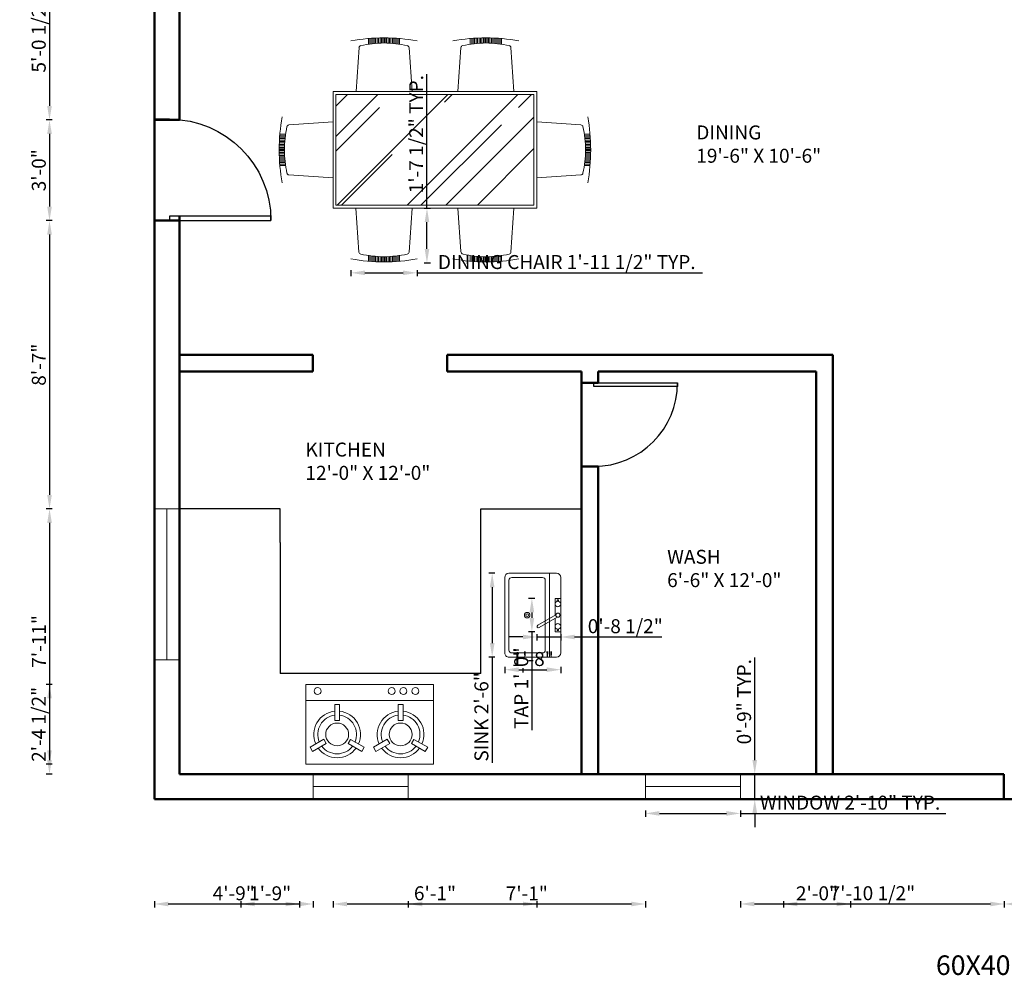
# Model space of a CAD drawing. Units: inches. Extents: x -46 to 764, y -530 to 112.
# Tile 1 of 5: x -46 to 307, y -530 to -188. Entities that reach past the tile are written whole.
import ezdxf

# ---------------------------------------------------------------- set-up
doc = ezdxf.new("R2010")
doc.units = ezdxf.units.IN
for name, color, linetype, lineweight in [('A-ANNO-DIMS', 2, 'Continuous', 18), ('A-AREA-IDEN', 7, 'Continuous', 18), ('A-DOOR', 3, 'Continuous', 25), ('A-EQPM', 9, 'Continuous', 18), ('A-FLOR-CASE', 32, 'Continuous', 25), ('A-FLOR-FIXT', 8, 'Continuous', 18), ('A-FURN-PATT', 252, 'Continuous', 13), ('A-GLAZ', 4, 'Continuous', 18), ('A-WALL', 7, 'Continuous', 50), ('furn', 28, 'Continuous', 18), ('txt', 167, 'Continuous', 18)]:
    doc.layers.add(name, color=color, linetype=linetype, lineweight=lineweight)
doc.styles.get("Standard").update_dxf_attribs({"font": 'arial.ttf'})
doc.dimstyles.new('ISO-25', dxfattribs={"dimtxt": 5, "dimasz": 5, "dimexe": 1.25, "dimexo": 0.625, "dimtad": 1, "dimlunit": 3, "dimtxsty": 'Standard', "dimcen": 2.5, "dimadec": 0, "dimazin": 0, "dimtfac": 1, "dimtmove": 0, "dimatfit": 3, "dimfxl": 1, "dimfxlon": 1, "dimarcsym": 0})

# ---------------------------------------------------------------- blocks, each defined once
blk = doc.blocks.new('*U2')
for p, q in [((0, 0), (0, -6)), ((40, 0), (40, -6))]:
    blk.add_line(p, q)
blk.add_lwpolyline([(0, 0), (0, 40), (1.75, 40), (1.75, 0)], close=True)
blk.add_arc((0, 0), 40, 0, 90)
blk = doc.blocks.new('Sink-single - 30 in top')
blk.add_line((-15, -3.999996), (15, -3.999996))
for points in [[(-13.5, 0), (13.5, 0)], [(-15, -18.499996), (-15, -1.5)], [(15, -1.5), (15, -18.499996)], [(-13.5, -17.499996), (-13.5, -6.499996)], [(-12.5, -5.499996), (12.5, -5.499996)], [(13.5, -6.499996), (13.5, -17.499996)], [(13.5, -19.999996), (-13.5, -19.999996)], [(12.5, -18.499996), (-12.5, -18.499996)]]:
    blk.add_lwpolyline(points)
for radius in [1, 0.5]:
    blk.add_circle((0, -11.999996), radius)
for centre, radius, start, end in [((-13.5, -1.5), 1.5, 90, 180), ((13.5, -1.5), 1.5, 0, 90), ((-12.5, -6.499996), 1, 90, 180), ((12.5, -6.499996), 1, 0, 90), ((-12.5, -17.499996), 1, 180, 270), ((12.5, -17.499996), 1, 270, 0), ((-13.5, -18.499996), 1.5, 180, 270), ((13.5, -18.499996), 1.5, 270, 0)]:
    blk.add_arc(centre, radius, start, end)
blk = doc.blocks.new('Faucet - kit sink top')
for p, q in [((-5.5, -0.75), (-5.5, -1.25)), ((-4.94278, -0.75), (-5.5, -0.75)), ((-5.5, -1.25), (-4.94278, -1.25)), ((-0.14775, -1.7441), (3.56698, -8.1782)), ((4.43301, -7.6782), (0.71828, -1.2441)), ((4.94278, -0.75), (5.5, -0.75)), ((5.5, -1.25), (4.94278, -1.25)), ((5.5, -0.75), (5.5, -1.25))]:
    blk.add_line(p, q)
blk.add_lwpolyline([(-0.00587, -2), (-6, -2), (-6, 0), (6, 0), (6, -2), (1.15195, -2)])
for centre, radius in [((-4, -1), 1), ((4, -1), 1), ((0, -1), 0.75)]:
    blk.add_circle(centre, radius)
blk.add_arc((4, -7.9282), 0.5, 210, 30)
blk = doc.blocks.new('CHAIR-DINING')
for p, q in [((1.8, 19.25), (2.87, 3.49)), ((21.83, 19.25), (20.76, 3.49)), ((6.22, 2.29), (6.22, 0.24)), ((6.74, 2.22), (6.74, 0.2)), ((7.26, 2.15), (7.26, 0.16)), ((7.78, 2.09), (7.78, 0.12)), ((8.3, 2.04), (8.3, 0.09)), ((8.83, 1.99), (8.83, 0.07)), ((9.35, 1.95), (9.35, 0.05)), ((9.87, 1.92), (9.87, 0.03)), ((10.39, 1.89), (10.39, 0.02)), ((10.91, 1.86), (10.91, 0.01)), ((11.43, 1.85), (11.43, 0)), ((11.82, 1.84), (11.82, 0)), ((12.21, 1.85), (12.21, 0)), ((12.73, 1.86), (12.73, 0.01)), ((13.25, 1.89), (13.25, 0.02)), ((13.77, 1.92), (13.77, 0.03)), ((14.29, 1.95), (14.29, 0.05)), ((14.81, 1.99), (14.81, 0.07)), ((15.33, 2.04), (15.33, 0.09)), ((15.85, 2.09), (15.85, 0.12)), ((16.37, 2.15), (16.37, 0.16)), ((16.89, 2.22), (16.89, 0.2)), ((17.41, 2.29), (17.41, 0.24))]:
    blk.add_line(p, q)
blk.add_lwpolyline([(0, 1.08, 0.091245), (23.64, 1.08, 0.091245)], format="xyb")
for centre, radius, start, end in [((3.65, 3.55), 0.781, 183.8745, 258.0355), ((12.57, 45.65), 43.82, 258.0355, 269.0138), ((11.06, 45.65), 43.82, 270.9862, 281.9645), ((19.99, 3.55), 0.781, 281.9645, 356.1255)]:
    blk.add_arc(centre, radius, start, end)
blk = doc.blocks.new('WIN-54IN')
blk.add_line((4.5, 54), (4.5, 0))
blk.add_lwpolyline([(0, 54), (9, 54), (9, 0), (0, 0)], close=True)
blk = doc.blocks.new('WIN-34IN')
blk.add_line((0, 4.5), (34, 4.5))
blk.add_lwpolyline([(0, 9), (34, 9), (34, 0), (0, 0)], close=True)
blk = doc.blocks.new('*D21')
at = {"layer": 'A-ANNO-DIMS', "color": 0, "lineweight": -2, "transparency": 16777216}
for p, q in [((178.25, -471.13), (178.25, -473.38)), ((212.25, -471.13), (212.25, -473.38)), ((183.25, -472.13), (207.25, -472.13)), ((212.25, -472.13), (285.66, -472.13))]:
    blk.add_line(p, q, dxfattribs=at)
at = {"layer": 'A-ANNO-DIMS', "color": 0, "transparency": 16777216}
for points in [[(183.25, -471.3), (183.25, -472.96), (178.25, -472.13)], [(207.25, -471.3), (207.25, -472.96), (212.25, -472.13)]]:
    blk.add_solid(points, dxfattribs=at)
at = {"layer": 'Defpoints', "color": 0, "transparency": 16777216}
for p in [(178.25, -467.03), (212.25, -467.03), (212.25, -472.13)]:
    blk.add_point(p, dxfattribs=at)
at = {"layer": 'A-ANNO-DIMS', "color": 0, "transparency": 16777216, "insert": (251.46, -468.92), "char_height": 5, "attachment_point": 5}
blk.add_mtext('WINDOW 2\'-10" TYP.', dxfattribs=at)
blk = doc.blocks.new('*D22')
at = {"layer": 'A-ANNO-DIMS', "color": 0, "lineweight": -2, "transparency": 16777216}
for p, q in [((217.35, -453.03), (217.35, -416.3)), ((216.35, -458.03), (218.6, -458.03)), ((217.35, -467.03), (217.35, -458.03)), ((216.35, -467.03), (218.6, -467.03)), ((217.35, -472.03), (217.35, -477.03))]:
    blk.add_line(p, q, dxfattribs=at)
at = {"layer": 'A-ANNO-DIMS', "color": 0, "transparency": 16777216}
for points in [[(216.52, -453.03), (218.19, -453.03), (217.35, -458.03)], [(216.52, -472.03), (218.19, -472.03), (217.35, -467.03)]]:
    blk.add_solid(points, dxfattribs=at)
at = {"layer": 'Defpoints', "color": 0, "transparency": 16777216}
for p in [(212.25, -458.03), (217.35, -458.03), (212.25, -467.03)]:
    blk.add_point(p, dxfattribs=at)
at = {"layer": 'A-ANNO-DIMS', "color": 0, "transparency": 16777216, "insert": (214.18, -432.17), "char_height": 5, "attachment_point": 5, "rotation": 90}
blk.add_mtext('0\'-9" TYP.', dxfattribs=at)
blk = doc.blocks.new('*D33')
at = {"layer": 'A-ANNO-DIMS', "color": 0, "lineweight": -2, "transparency": 16777216}
for p, q in [((72.94, -277.73), (72.94, -279.98)), ((96.58, -277.73), (96.58, -279.98)), ((77.94, -278.73), (91.58, -278.73)), ((96.58, -278.73), (198.65, -278.73))]:
    blk.add_line(p, q, dxfattribs=at)
at = {"layer": 'A-ANNO-DIMS', "color": 0, "transparency": 16777216}
for points in [[(77.94, -277.9), (77.94, -279.57), (72.94, -278.73)], [(91.58, -277.9), (91.58, -279.57), (96.58, -278.73)]]:
    blk.add_solid(points, dxfattribs=at)
at = {"layer": 'Defpoints', "color": 0, "transparency": 16777216}
for p in [(72.94, -275.19), (96.58, -275.19), (96.58, -278.73)]:
    blk.add_point(p, dxfattribs=at)
at = {"layer": 'A-ANNO-DIMS', "color": 0, "transparency": 16777216, "insert": (150.12, -275.52), "char_height": 5, "attachment_point": 5}
blk.add_mtext('DINING CHAIR 1\'-11 1/2" TYP.', dxfattribs=at)
blk = doc.blocks.new('*D34')
at = {"layer": 'A-ANNO-DIMS', "color": 0, "lineweight": -2, "transparency": 16777216}
for p, q in [((100.12, -255.58), (100.12, -207.67)), ((99.12, -255.58), (101.37, -255.58)), ((100.12, -270.19), (100.12, -260.58)), ((99.12, -275.19), (101.37, -275.19))]:
    blk.add_line(p, q, dxfattribs=at)
at = {"layer": 'A-ANNO-DIMS', "color": 0, "transparency": 16777216}
for points in [[(99.29, -260.58), (100.96, -260.58), (100.12, -255.58)], [(99.29, -270.19), (100.96, -270.19), (100.12, -275.19)]]:
    blk.add_solid(points, dxfattribs=at)
at = {"layer": 'Defpoints', "color": 0, "transparency": 16777216}
for p in [(96.58, -255.58), (100.12, -255.58), (96.58, -275.19)]:
    blk.add_point(p, dxfattribs=at)
at = {"layer": 'A-ANNO-DIMS', "color": 0, "transparency": 16777216, "insert": (96.91, -229.12), "char_height": 5, "attachment_point": 5, "rotation": 90}
blk.add_mtext('1\'-7 1/2" TYP.', dxfattribs=at)
blk = doc.blocks.new('*D35')
at = {"layer": 'A-ANNO-DIMS', "color": 0, "lineweight": -2, "transparency": 16777216}
for p, q in [((124.45, -386.21), (122.2, -386.21)), ((123.45, -391.21), (123.45, -411.21)), ((124.45, -416.21), (122.2, -416.21)), ((123.45, -416.21), (123.45, -453.97))]:
    blk.add_line(p, q, dxfattribs=at)
at = {"layer": 'A-ANNO-DIMS', "color": 0, "transparency": 16777216}
for points in [[(122.62, -391.21), (124.28, -391.21), (123.45, -386.21)], [(122.62, -411.21), (124.28, -411.21), (123.45, -416.21)]]:
    blk.add_solid(points, dxfattribs=at)
at = {"layer": 'Defpoints', "color": 0, "transparency": 16777216}
for p in [(127.95, -386.21), (123.45, -416.21), (127.95, -416.21)]:
    blk.add_point(p, dxfattribs=at)
at = {"layer": 'A-ANNO-DIMS', "color": 0, "transparency": 16777216, "insert": (120.24, -437.59), "char_height": 5, "attachment_point": 5, "rotation": 90}
blk.add_mtext('SINK 2\'-6"', dxfattribs=at)
blk = doc.blocks.new('*D36')
at = {"layer": 'A-ANNO-DIMS', "color": 0, "lineweight": -2, "transparency": 16777216}
for p, q in [((127.95, -419.71), (127.95, -421.96)), ((132.95, -420.71), (142.95, -420.71)), ((147.95, -419.71), (147.95, -421.96))]:
    blk.add_line(p, q, dxfattribs=at)
at = {"layer": 'A-ANNO-DIMS', "color": 0, "transparency": 16777216}
for points in [[(132.95, -419.87), (132.95, -421.54), (127.95, -420.71)], [(142.95, -419.87), (142.95, -421.54), (147.95, -420.71)]]:
    blk.add_solid(points, dxfattribs=at)
at = {"layer": 'Defpoints', "color": 0, "transparency": 16777216}
for p in [(127.95, -416.21), (147.95, -416.21), (147.95, -420.71)]:
    blk.add_point(p, dxfattribs=at)
at = {"layer": 'A-ANNO-DIMS', "color": 0, "transparency": 16777216, "insert": (137.95, -417.53), "char_height": 5, "attachment_point": 5}
blk.add_mtext('1\'-8"', dxfattribs=at)
blk = doc.blocks.new('*D37')
at = {"layer": 'A-ANNO-DIMS', "color": 0, "lineweight": -2, "transparency": 16777216}
for p, q in [((138.65, -395.21), (136.4, -395.21)), ((137.65, -400.21), (137.65, -402.21)), ((138.65, -407.21), (136.4, -407.21)), ((137.65, -407.21), (137.65, -442.4))]:
    blk.add_line(p, q, dxfattribs=at)
at = {"layer": 'A-ANNO-DIMS', "color": 0, "transparency": 16777216}
for points in [[(136.82, -400.21), (138.48, -400.21), (137.65, -395.21)], [(136.82, -402.21), (138.48, -402.21), (137.65, -407.21)]]:
    blk.add_solid(points, dxfattribs=at)
at = {"layer": 'Defpoints', "color": 0, "transparency": 16777216}
for p in [(139.45, -395.21), (137.65, -407.21), (139.45, -407.21)]:
    blk.add_point(p, dxfattribs=at)
at = {"layer": 'A-ANNO-DIMS', "color": 0, "transparency": 16777216, "insert": (134.47, -427.3), "char_height": 5, "attachment_point": 5, "rotation": 90}
blk.add_mtext('TAP 1\'-0"', dxfattribs=at)
blk = doc.blocks.new('*D38')
at = {"layer": 'A-ANNO-DIMS', "color": 0, "lineweight": -2, "transparency": 16777216}
for p, q in [((139.45, -408.01), (139.45, -410.26)), ((147.95, -408.01), (147.95, -410.26)), ((134.45, -409.01), (129.45, -409.01)), ((139.45, -409.01), (147.95, -409.01)), ((152.95, -409.01), (184.14, -409.01))]:
    blk.add_line(p, q, dxfattribs=at)
at = {"layer": 'A-ANNO-DIMS', "color": 0, "transparency": 16777216}
for points in [[(134.45, -408.17), (134.45, -409.84), (139.45, -409.01)], [(152.95, -408.17), (152.95, -409.84), (147.95, -409.01)]]:
    blk.add_solid(points, dxfattribs=at)
at = {"layer": 'Defpoints', "color": 0, "transparency": 16777216}
for p in [(139.45, -407.21), (147.95, -407.21), (147.95, -409.01)]:
    blk.add_point(p, dxfattribs=at)
at = {"layer": 'A-ANNO-DIMS', "color": 0, "transparency": 16777216, "insert": (171.05, -405.8), "char_height": 5, "attachment_point": 5}
blk.add_mtext('0\'-8 1/2"', dxfattribs=at)
blk = doc.blocks.new('*D43')
at = {"layer": 'A-ANNO-DIMS', "color": 0, "lineweight": -2, "transparency": 16777216}
for p, q in [((227.62, -503.53), (227.62, -505.78)), ((251.62, -503.53), (251.62, -505.78)), ((232.62, -504.53), (246.62, -504.53))]:
    blk.add_line(p, q, dxfattribs=at)
at = {"layer": 'A-ANNO-DIMS', "color": 0, "transparency": 16777216}
for points in [[(232.62, -503.7), (232.62, -505.36), (227.62, -504.53)], [(246.62, -503.7), (246.62, -505.36), (251.62, -504.53)]]:
    blk.add_solid(points, dxfattribs=at)
at = {"layer": 'Defpoints', "color": 0, "transparency": 16777216}
for p in [(227.62, -105.31), (251.62, -105.31), (251.62, -504.53)]:
    blk.add_point(p, dxfattribs=at)
at = {"layer": 'A-ANNO-DIMS', "color": 0, "transparency": 16777216, "insert": (239.62, -501.35), "char_height": 5, "attachment_point": 5}
blk.add_mtext('2\'-0"', dxfattribs=at)
blk = doc.blocks.new('*D55')
at = {"layer": 'A-ANNO-DIMS', "color": 0, "lineweight": -2, "transparency": 16777216}
for p, q in [((-33.88, -163.31), (-36.13, -163.31)), ((-34.88, -168.31), (-34.88, -219.03)), ((-33.88, -224.03), (-36.13, -224.03))]:
    blk.add_line(p, q, dxfattribs=at)
at = {"layer": 'A-ANNO-DIMS', "color": 0, "transparency": 16777216}
for points in [[(-35.71, -168.31), (-34.04, -168.31), (-34.88, -163.31)], [(-35.71, -219.03), (-34.04, -219.03), (-34.88, -224.03)]]:
    blk.add_solid(points, dxfattribs=at)
at = {"layer": 'Defpoints', "color": 0, "transparency": 16777216}
for p in [(2.62, -163.31), (-34.88, -224.03), (2.62, -224.03)]:
    blk.add_point(p, dxfattribs=at)
at = {"layer": 'A-ANNO-DIMS', "color": 0, "transparency": 16777216, "insert": (-38.09, -193.67), "char_height": 5, "attachment_point": 5, "rotation": 90}
blk.add_mtext('5\'-0 1/2"', dxfattribs=at)
blk = doc.blocks.new('*D56')
at = {"layer": 'A-ANNO-DIMS', "color": 0, "lineweight": -2, "transparency": 16777216}
for p, q in [((-33.88, -224.03), (-36.13, -224.03)), ((-34.88, -229.03), (-34.88, -255.03)), ((-33.88, -260.03), (-36.13, -260.03))]:
    blk.add_line(p, q, dxfattribs=at)
at = {"layer": 'A-ANNO-DIMS', "color": 0, "transparency": 16777216}
for points in [[(-35.71, -229.03), (-34.04, -229.03), (-34.88, -224.03)], [(-35.71, -255.03), (-34.04, -255.03), (-34.88, -260.03)]]:
    blk.add_solid(points, dxfattribs=at)
at = {"layer": 'Defpoints', "color": 0, "transparency": 16777216}
for p in [(2.62, -224.03), (-34.88, -260.03), (2.62, -260.03)]:
    blk.add_point(p, dxfattribs=at)
at = {"layer": 'A-ANNO-DIMS', "color": 0, "transparency": 16777216, "insert": (-38.06, -242.03), "char_height": 5, "attachment_point": 5, "rotation": 90}
blk.add_mtext('3\'-0"', dxfattribs=at)
blk = doc.blocks.new('*D57')
at = {"layer": 'A-ANNO-DIMS', "color": 0, "lineweight": -2, "transparency": 16777216}
for p, q in [((-33.88, -260.03), (-36.13, -260.03)), ((-34.88, -265.03), (-34.88, -358.17)), ((-33.88, -363.17), (-36.13, -363.17))]:
    blk.add_line(p, q, dxfattribs=at)
at = {"layer": 'A-ANNO-DIMS', "color": 0, "transparency": 16777216}
for points in [[(-35.71, -265.03), (-34.04, -265.03), (-34.88, -260.03)], [(-35.71, -358.17), (-34.04, -358.17), (-34.88, -363.17)]]:
    blk.add_solid(points, dxfattribs=at)
at = {"layer": 'Defpoints', "color": 0, "transparency": 16777216}
for p in [(2.62, -260.03), (-34.88, -363.17), (2.62, -363.17)]:
    blk.add_point(p, dxfattribs=at)
at = {"layer": 'A-ANNO-DIMS', "color": 0, "transparency": 16777216, "insert": (-38.05, -311.6), "char_height": 5, "attachment_point": 5, "rotation": 90}
blk.add_mtext('8\'-7"', dxfattribs=at)
blk = doc.blocks.new('*D62')
at = {"layer": 'A-ANNO-DIMS', "color": 0, "lineweight": -2, "transparency": 16777216}
for p, q in [((2.62, -503.53), (2.62, -505.78)), ((59.41, -503.53), (59.41, -505.78)), ((7.62, -504.53), (54.41, -504.53))]:
    blk.add_line(p, q, dxfattribs=at)
at = {"layer": 'A-ANNO-DIMS', "color": 0, "transparency": 16777216}
for points in [[(7.62, -503.7), (7.62, -505.36), (2.62, -504.53)], [(54.41, -503.7), (54.41, -505.36), (59.41, -504.53)]]:
    blk.add_solid(points, dxfattribs=at)
at = {"layer": 'Defpoints', "color": 0, "transparency": 16777216}
for p in [(2.62, -467.03), (59.41, -467.03), (59.41, -504.53)]:
    blk.add_point(p, dxfattribs=at)
at = {"layer": 'A-ANNO-DIMS', "color": 0, "transparency": 16777216, "insert": (31.02, -501.35), "char_height": 5, "attachment_point": 5}
blk.add_mtext('4\'-9"', dxfattribs=at)
blk = doc.blocks.new('*D63')
at = {"layer": 'A-ANNO-DIMS', "color": 0, "lineweight": -2, "transparency": 16777216}
for p, q in [((93.41, -503.53), (93.41, -505.78)), ((178.25, -503.53), (178.25, -505.78)), ((98.41, -504.53), (173.25, -504.53))]:
    blk.add_line(p, q, dxfattribs=at)
at = {"layer": 'A-ANNO-DIMS', "color": 0, "transparency": 16777216}
for points in [[(98.41, -503.7), (98.41, -505.36), (93.41, -504.53)], [(173.25, -503.7), (173.25, -505.36), (178.25, -504.53)]]:
    blk.add_solid(points, dxfattribs=at)
at = {"layer": 'Defpoints', "color": 0, "transparency": 16777216}
for p in [(93.41, -467.03), (178.25, -467.03), (178.25, -504.53)]:
    blk.add_point(p, dxfattribs=at)
at = {"layer": 'A-ANNO-DIMS', "color": 0, "transparency": 16777216, "insert": (135.83, -501.39), "char_height": 5, "attachment_point": 5}
blk.add_mtext('7\'-1"', dxfattribs=at)
blk = doc.blocks.new('*D64')
at = {"layer": 'A-ANNO-DIMS', "color": 0, "lineweight": -2, "transparency": 16777216}
for p, q in [((212.25, -503.53), (212.25, -505.78)), ((306.62, -503.53), (306.62, -505.78)), ((217.25, -504.53), (301.62, -504.53))]:
    blk.add_line(p, q, dxfattribs=at)
at = {"layer": 'A-ANNO-DIMS', "color": 0, "transparency": 16777216}
for points in [[(217.25, -503.7), (217.25, -505.36), (212.25, -504.53)], [(301.62, -503.7), (301.62, -505.36), (306.62, -504.53)]]:
    blk.add_solid(points, dxfattribs=at)
at = {"layer": 'Defpoints', "color": 0, "transparency": 16777216}
for p in [(212.25, -467.03), (306.62, -467.03), (306.62, -504.53)]:
    blk.add_point(p, dxfattribs=at)
at = {"layer": 'A-ANNO-DIMS', "color": 0, "transparency": 16777216, "insert": (259.43, -501.32), "char_height": 5, "attachment_point": 5}
blk.add_mtext('7\'-10 1/2"', dxfattribs=at)
blk = doc.blocks.new('*D65')
at = {"layer": 'A-ANNO-DIMS', "color": 0, "lineweight": -2, "transparency": 16777216}
for p, q in [((306.62, -503.53), (306.62, -505.78)), ((340.48, -503.53), (340.48, -505.78)), ((311.62, -504.53), (335.48, -504.53))]:
    blk.add_line(p, q, dxfattribs=at)
at = {"layer": 'A-ANNO-DIMS', "color": 0, "transparency": 16777216}
for points in [[(311.62, -503.7), (311.62, -505.36), (306.62, -504.53)], [(335.48, -503.7), (335.48, -505.36), (340.48, -504.53)]]:
    blk.add_solid(points, dxfattribs=at)
at = {"layer": 'Defpoints', "color": 0, "transparency": 16777216}
for p in [(306.62, -467.03), (340.48, -467.03), (340.48, -504.53)]:
    blk.add_point(p, dxfattribs=at)
at = {"layer": 'A-ANNO-DIMS', "color": 0, "transparency": 16777216, "insert": (323.55, -501.35), "char_height": 5, "attachment_point": 5}
blk.add_mtext('2\'-10"', dxfattribs=at)
blk = doc.blocks.new('*D68')
at = {"layer": 'A-ANNO-DIMS', "color": 0, "lineweight": -2, "transparency": 16777216}
for p, q in [((2.62, 100.72), (2.62, 102.97)), ((11.62, 100.72), (11.62, 102.97)), ((-2.38, 101.72), (-21.92, 101.72)), ((11.62, 101.72), (2.62, 101.72)), ((16.62, 101.72), (21.62, 101.72))]:
    blk.add_line(p, q, dxfattribs=at)
at = {"layer": 'A-ANNO-DIMS', "color": 0, "transparency": 16777216}
for points in [[(-2.38, 102.55), (-2.38, 100.88), (2.62, 101.72)], [(16.62, 102.55), (16.62, 100.88), (11.62, 101.72)]]:
    blk.add_solid(points, dxfattribs=at)
at = {"layer": 'Defpoints', "color": 0, "transparency": 16777216}
for p in [(2.62, 101.72), (11.62, -458.03), (2.62, -467.03)]:
    blk.add_point(p, dxfattribs=at)
at = {"layer": 'A-ANNO-DIMS', "color": 0, "transparency": 16777216, "insert": (-14.65, 104.89), "char_height": 5, "attachment_point": 5}
blk.add_mtext('0\'-9"', dxfattribs=at)
blk = doc.blocks.new('*D69')
at = {"layer": 'A-ANNO-DIMS', "color": 0, "lineweight": -2, "transparency": 16777216}
for p, q in [((155.34, 100.72), (155.34, 102.97)), ((161.34, 100.72), (161.34, 102.97)), ((150.34, 101.72), (145.34, 101.72)), ((155.34, 101.72), (161.34, 101.72)), ((166.34, 101.72), (185.88, 101.72))]:
    blk.add_line(p, q, dxfattribs=at)
at = {"layer": 'A-ANNO-DIMS', "color": 0, "transparency": 16777216}
for points in [[(150.34, 102.55), (150.34, 100.88), (155.34, 101.72)], [(166.34, 102.55), (166.34, 100.88), (161.34, 101.72)]]:
    blk.add_solid(points, dxfattribs=at)
at = {"layer": 'Defpoints', "color": 0, "transparency": 16777216}
for p in [(161.34, 101.72), (155.34, -458.03), (161.34, -458.03)]:
    blk.add_point(p, dxfattribs=at)
at = {"layer": 'A-ANNO-DIMS', "color": 0, "transparency": 16777216, "insert": (178.61, 104.89), "char_height": 5, "attachment_point": 5}
blk.add_mtext('0\'-6"', dxfattribs=at)
blk = doc.blocks.new('*D70')
at = {"layer": 'A-ANNO-DIMS', "color": 0, "lineweight": -2, "transparency": 16777216}
for p, q in [((59.34, 100.72), (59.34, 102.97)), ((107.34, 100.72), (107.34, 102.97)), ((64.34, 101.72), (102.34, 101.72))]:
    blk.add_line(p, q, dxfattribs=at)
at = {"layer": 'A-ANNO-DIMS', "color": 0, "transparency": 16777216}
for points in [[(64.34, 102.55), (64.34, 100.88), (59.34, 101.72)], [(102.34, 102.55), (102.34, 100.88), (107.34, 101.72)]]:
    blk.add_solid(points, dxfattribs=at)
at = {"layer": 'Defpoints', "color": 0, "transparency": 16777216}
for p in [(107.34, 101.72), (59.34, -308.03), (107.34, -308.03)]:
    blk.add_point(p, dxfattribs=at)
at = {"layer": 'A-ANNO-DIMS', "color": 0, "transparency": 16777216, "insert": (83.34, 104.89), "char_height": 5, "attachment_point": 5}
blk.add_mtext('4\'-0"', dxfattribs=at)
blk = doc.blocks.new('*D71')
at = {"layer": 'A-ANNO-DIMS', "color": 0, "lineweight": -2, "transparency": 16777216}
for p, q in [((47.62, 100.72), (47.62, 102.97)), ((119.34, 100.72), (119.34, 102.97)), ((52.62, 101.72), (114.34, 101.72))]:
    blk.add_line(p, q, dxfattribs=at)
at = {"layer": 'A-ANNO-DIMS', "color": 0, "transparency": 16777216}
for points in [[(52.62, 102.55), (52.62, 100.88), (47.62, 101.72)], [(114.34, 102.55), (114.34, 100.88), (119.34, 101.72)]]:
    blk.add_solid(points, dxfattribs=at)
at = {"layer": 'Defpoints', "color": 0, "transparency": 16777216}
for p in [(119.34, 101.72), (47.62, -422.03), (119.34, -422.03)]:
    blk.add_point(p, dxfattribs=at)
at = {"layer": 'A-ANNO-DIMS', "color": 0, "transparency": 16777216, "insert": (83.48, 104.93), "char_height": 5, "attachment_point": 5}
blk.add_mtext('5\'-11 1/2"', dxfattribs=at)
blk = doc.blocks.new('*D72')
at = {"layer": 'A-ANNO-DIMS', "color": 0, "lineweight": -2, "transparency": 16777216}
for p, q in [((11.62, 100.72), (11.62, 102.97)), ((47.62, 100.72), (47.62, 102.97)), ((16.62, 101.72), (42.62, 101.72))]:
    blk.add_line(p, q, dxfattribs=at)
at = {"layer": 'A-ANNO-DIMS', "color": 0, "transparency": 16777216}
for points in [[(16.62, 102.55), (16.62, 100.88), (11.62, 101.72)], [(42.62, 102.55), (42.62, 100.88), (47.62, 101.72)]]:
    blk.add_solid(points, dxfattribs=at)
at = {"layer": 'Defpoints', "color": 0, "transparency": 16777216}
for p in [(47.62, 101.72), (11.62, -363.17), (47.62, -363.17)]:
    blk.add_point(p, dxfattribs=at)
at = {"layer": 'A-ANNO-DIMS', "color": 0, "transparency": 16777216, "insert": (29.62, 104.9), "char_height": 5, "attachment_point": 5}
blk.add_mtext('3\'-0"', dxfattribs=at)
blk = doc.blocks.new('*D73')
at = {"layer": 'A-ANNO-DIMS', "color": 0, "lineweight": -2, "transparency": 16777216}
for p, q in [((-33.88, -363.17), (-36.13, -363.17)), ((-34.88, -368.17), (-34.88, -453.03)), ((-33.88, -458.03), (-36.13, -458.03))]:
    blk.add_line(p, q, dxfattribs=at)
at = {"layer": 'A-ANNO-DIMS', "color": 0, "transparency": 16777216}
for points in [[(-35.71, -368.17), (-34.04, -368.17), (-34.88, -363.17)], [(-35.71, -453.03), (-34.04, -453.03), (-34.88, -458.03)]]:
    blk.add_solid(points, dxfattribs=at)
at = {"layer": 'Defpoints', "color": 0, "transparency": 16777216}
for p in [(11.62, -363.17), (-34.88, -458.03), (11.62, -458.03)]:
    blk.add_point(p, dxfattribs=at)
at = {"layer": 'A-ANNO-DIMS', "color": 0, "transparency": 16777216, "insert": (-38.01, -410.6), "char_height": 5, "attachment_point": 5, "rotation": 90}
blk.add_mtext('7\'-11"', dxfattribs=at)
blk = doc.blocks.new('*D74')
at = {"layer": 'A-ANNO-DIMS', "color": 0, "lineweight": -2, "transparency": 16777216}
for p, q in [((56.83, 100.72), (56.83, 102.97)), ((102.5, 100.72), (102.5, 102.97)), ((61.83, 101.72), (97.5, 101.72))]:
    blk.add_line(p, q, dxfattribs=at)
at = {"layer": 'A-ANNO-DIMS', "color": 0, "transparency": 16777216}
for points in [[(61.83, 102.55), (61.83, 100.88), (56.83, 101.72)], [(97.5, 102.55), (97.5, 100.88), (102.5, 101.72)]]:
    blk.add_solid(points, dxfattribs=at)
at = {"layer": 'Defpoints', "color": 0, "transparency": 16777216}
for p in [(102.5, 101.72), (56.83, -426), (102.5, -426)]:
    blk.add_point(p, dxfattribs=at)
at = {"layer": 'A-ANNO-DIMS', "color": 0, "transparency": 16777216, "insert": (79.66, 104.93), "char_height": 5, "attachment_point": 5}
blk.add_mtext('3\'-9 1/2"', dxfattribs=at)
blk = doc.blocks.new('*D75')
at = {"layer": 'A-ANNO-DIMS', "color": 0, "lineweight": -2, "transparency": 16777216}
for p, q in [((-33.88, -426), (-36.13, -426)), ((-34.88, -431), (-34.88, -449.54)), ((-33.88, -454.54), (-36.13, -454.54))]:
    blk.add_line(p, q, dxfattribs=at)
at = {"layer": 'A-ANNO-DIMS', "color": 0, "transparency": 16777216}
for points in [[(-35.71, -431), (-34.04, -431), (-34.88, -426)], [(-35.71, -449.54), (-34.04, -449.54), (-34.88, -454.54)]]:
    blk.add_solid(points, dxfattribs=at)
at = {"layer": 'Defpoints', "color": 0, "transparency": 16777216}
for p in [(56.83, -426), (-34.88, -454.54), (56.83, -454.54)]:
    blk.add_point(p, dxfattribs=at)
at = {"layer": 'A-ANNO-DIMS', "color": 0, "transparency": 16777216, "insert": (-38.09, -440.27), "char_height": 5, "attachment_point": 5, "rotation": 90}
blk.add_mtext('2\'-4 1/2"', dxfattribs=at)
blk = doc.blocks.new('*D78')
at = {"layer": 'A-ANNO-DIMS', "color": 0, "lineweight": -2, "transparency": 16777216}
for p, q in [((245.34, 100.72), (245.34, 102.97)), ((401.62, 100.72), (401.62, 102.97)), ((250.34, 101.72), (396.62, 101.72))]:
    blk.add_line(p, q, dxfattribs=at)
at = {"layer": 'A-ANNO-DIMS', "color": 0, "transparency": 16777216}
for points in [[(250.34, 102.55), (250.34, 100.88), (245.34, 101.72)], [(396.62, 102.55), (396.62, 100.88), (401.62, 101.72)]]:
    blk.add_solid(points, dxfattribs=at)
at = {"layer": 'Defpoints', "color": 0, "transparency": 16777216}
for p in [(401.62, 101.72), (245.34, -458.03), (401.62, -458.03)]:
    blk.add_point(p, dxfattribs=at)
at = {"layer": 'A-ANNO-DIMS', "color": 0, "transparency": 16777216, "insert": (323.48, 104.93), "char_height": 5, "attachment_point": 5}
blk.add_mtext('13\'-0 1/2"', dxfattribs=at)
blk = doc.blocks.new('*D80')
at = {"layer": 'A-ANNO-DIMS', "color": 0, "lineweight": -2, "transparency": 16777216}
for p, q in [((66.53, -503.53), (66.53, -505.78)), ((139.44, -503.53), (139.44, -505.78)), ((71.53, -504.53), (134.44, -504.53))]:
    blk.add_line(p, q, dxfattribs=at)
at = {"layer": 'A-ANNO-DIMS', "color": 0, "transparency": 16777216}
for points in [[(71.53, -503.7), (71.53, -505.36), (66.53, -504.53)], [(134.44, -503.7), (134.44, -505.36), (139.44, -504.53)]]:
    blk.add_solid(points, dxfattribs=at)
at = {"layer": 'Defpoints', "color": 0, "transparency": 16777216}
for p in [(66.53, -255.58), (139.44, -255.58), (139.44, -504.53)]:
    blk.add_point(p, dxfattribs=at)
at = {"layer": 'A-ANNO-DIMS', "color": 0, "transparency": 16777216, "insert": (102.99, -501.35), "char_height": 5, "attachment_point": 5}
blk.add_mtext('6\'-1"', dxfattribs=at)
blk = doc.blocks.new('*D81')
at = {"layer": 'A-ANNO-DIMS', "color": 0, "lineweight": -2, "transparency": 16777216}
for p, q in [((759.12, -213.92), (761.37, -213.92)), ((760.12, -218.92), (760.12, -250.58)), ((759.12, -255.58), (761.37, -255.58))]:
    blk.add_line(p, q, dxfattribs=at)
at = {"layer": 'A-ANNO-DIMS', "color": 0, "transparency": 16777216}
for points in [[(759.29, -218.92), (760.96, -218.92), (760.12, -213.92)], [(759.29, -250.58), (760.96, -250.58), (760.12, -255.58)]]:
    blk.add_solid(points, dxfattribs=at)
at = {"layer": 'Defpoints', "color": 0, "transparency": 16777216}
for p in [(139.44, -213.92), (139.44, -255.58), (760.12, -255.58)]:
    blk.add_point(p, dxfattribs=at)
at = {"layer": 'A-ANNO-DIMS', "color": 0, "transparency": 16777216, "insert": (756.91, -234.75), "char_height": 5, "attachment_point": 5, "rotation": 90}
blk.add_mtext('3\'-5 1/2"', dxfattribs=at)
blk = doc.blocks.new('*D82')
at = {"layer": 'A-ANNO-DIMS', "color": 0, "lineweight": -2, "transparency": 16777216}
for p, q in [((33.53, -503.53), (33.53, -505.78)), ((54.53, -503.53), (54.53, -505.78)), ((38.53, -504.53), (49.53, -504.53))]:
    blk.add_line(p, q, dxfattribs=at)
at = {"layer": 'A-ANNO-DIMS', "color": 0, "transparency": 16777216}
for points in [[(38.53, -503.7), (38.53, -505.36), (33.53, -504.53)], [(49.53, -503.7), (49.53, -505.36), (54.53, -504.53)]]:
    blk.add_solid(points, dxfattribs=at)
at = {"layer": 'Defpoints', "color": 0, "transparency": 16777216}
for p in [(33.53, -3.78), (54.53, -3.78), (54.53, -504.53)]:
    blk.add_point(p, dxfattribs=at)
at = {"layer": 'A-ANNO-DIMS', "color": 0, "transparency": 16777216, "insert": (44.03, -501.35), "char_height": 5, "attachment_point": 5}
blk.add_mtext('1\'-9"', dxfattribs=at)

msp = doc.modelspace()

# ---------------------------------------------------------------- hatches: boundary and pattern name
at = {"layer": 'A-FURN-PATT'}
h = msp.add_hatch(dxfattribs=at)
h.set_pattern_fill('AR-RROOF', color=256, scale=1.041506, angle=45, style=0)
h.set_pattern_definition([(45, (-1846.616, -1123.131), (22.44717, 59.8591), [396.8136, -52.9085, 132.2712, -26.4542]), (45, (-1831.09, -1088.9), (-43.5849, 6.17297), [79.3627, -8.7299, 158.7254, -19.8407]), (45, (-1853.163, -1097.878), (84.73806, 109.80406), [211.6339, -37.036, 105.817, -26.4542])])
h.paths.add_polyline_path([(67.574, -214.957), (67.574, -254.534), (138.397, -254.534), (138.397, -214.957)])

# ---------------------------------------------------------------- linework, layer by layer
at = {"layer": 'A-EQPM'}
for p, q in [((56.834, -426.004), (102.496, -426.004)), ((56.834, -426.004), (56.834, -454.543)), ((102.496, -426.004), (102.496, -454.543)), ((56.834, -431.712), (102.496, -431.712)), ((67.148, -438.868), (67.15, -433.18)), ((67.15, -433.18), (68.863, -433.18)), ((68.861, -438.868), (68.863, -433.18)), ((89.84, -438.868), (89.843, -433.18)), ((89.843, -433.18), (91.555, -433.18)), ((91.553, -438.868), (91.555, -433.18)), ((67.148, -438.868), (68.861, -438.868)), ((89.84, -438.868), (91.553, -438.868)), ((63.247, -445.62), (58.319, -448.462)), ((64.102, -447.103), (59.175, -449.946)), ((64.102, -447.103), (63.247, -445.62)), ((72.757, -445.624), (71.901, -447.106)), ((71.901, -447.106), (76.826, -449.952)), ((72.757, -445.624), (77.682, -448.47)), ((85.939, -445.62), (81.011, -448.462)), ((86.794, -447.103), (81.867, -449.946)), ((86.794, -447.103), (85.939, -445.62)), ((95.45, -445.624), (94.593, -447.106)), ((94.593, -447.106), (99.518, -449.952)), ((95.45, -445.624), (100.375, -448.47)), ((59.175, -449.946), (58.319, -448.462)), ((77.682, -448.47), (76.826, -449.952)), ((81.867, -449.946), (81.011, -448.462)), ((100.375, -448.47), (99.518, -449.952)), ((56.834, -454.543), (102.496, -454.543))]:
    msp.add_line(p, q, dxfattribs=at)
at = {"layer": 'A-EQPM', "extrusion": (0, 0, -1)}
for centre, major_axis, start_param, end_param in [((61.006, -428.341), (0.876, -0.876), 2.3561945, 8.6393798), ((87.512, -428.341), (0.876, -0.876), 2.3561945, 8.6393798), ((91.707, -428.341), (0.876, -0.876), 2.3561945, 8.6393798), ((95.997, -428.341), (0.876, -0.876), 2.3561945, 8.6393798), ((68.003, -443.865), (-0.011, -8.363), 1.1487904, 3.0380671), ((68.003, -443.865), (-0.003, -8.363), 3.2441732, 5.1334499), ((90.695, -443.865), (-0.012, -8.363), 1.148752, 3.0380287), ((90.695, -443.865), (0.005, -8.363), 3.2450997, 5.1343764), ((68.003, -443.865), (-4.904, -4.904), 0.385932, 2.2328101), ((68.003, -443.865), (2.886, -2.886), 2.3561945, 8.6393798), ((68.003, -443.865), (-4.904, -4.904), 2.4803271, 4.3272052), ((90.695, -443.865), (-4.904, -4.904), 0.385932, 2.2328101), ((90.695, -443.865), (2.886, -2.886), 2.3561945, 8.6393798), ((90.695, -443.865), (4.904, -4.904), 4.0511235, 5.8980015), ((68.003, -443.865), (0.002, -8.363), -0.9440105, 0.9452662), ((68.003, -443.865), (4.904, -4.904), 6.1455186, 7.9923966), ((90.695, -443.865), (0.014, -8.363), -0.9425843, 0.9466925), ((90.695, -443.865), (4.904, -4.904), 6.1455186, 7.9923966)]:
    msp.add_ellipse(centre, major_axis=major_axis, ratio=1, start_param=start_param, end_param=end_param, dxfattribs=at)
at = {"layer": 'A-FLOR-CASE'}
for p, q in [((47.624, -363.167), (11.624, -363.167)), ((47.624, -375.167), (47.624, -363.167)), ((119.339, -363.167), (155.339, -363.167)), ((119.339, -375.167), (119.339, -363.167)), ((47.624, -375.167), (47.624, -422.03)), ((119.339, -422.03), (119.339, -375.167)), ((119.339, -422.03), (47.624, -422.03))]:
    msp.add_line(p, q, dxfattribs=at)
at = {"layer": 'A-WALL'}
for p, q in [((2.624, -467.03), (2.624, 12.97)), ((11.624, -224.03), (11.624, 3.97)), ((11.624, -224.03), (2.624, -224.03)), ((11.624, -260.03), (2.624, -260.03)), ((11.624, -458.03), (11.624, -258.443)), ((59.339, -308.03), (11.624, -308.03)), ((59.339, -314.03), (59.339, -308.03)), ((155.339, -308.03), (107.339, -308.03)), ((107.339, -314.03), (107.339, -308.03)), ((155.339, -308.03), (161.339, -308.03)), ((161.339, -308.03), (239.339, -308.03)), ((239.339, -308.03), (245.339, -308.03)), ((245.339, -308.03), (245.339, -458.03)), ((59.339, -314.03), (11.624, -314.03)), ((155.339, -314.03), (107.339, -314.03)), ((155.339, -458.03), (155.339, -314.03)), ((161.339, -314.03), (239.339, -314.03)), ((161.339, -318.03), (161.339, -314.03)), ((239.339, -314.03), (239.339, -458.03)), ((155.339, -318.03), (161.339, -318.03)), ((155.339, -348.03), (161.339, -348.03)), ((161.339, -458.03), (161.339, -348.03)), ((306.481, -458.03), (11.624, -458.03)), ((306.481, -458.03), (306.481, -467.03)), ((722.624, -467.03), (2.624, -467.03))]:
    msp.add_line(p, q, dxfattribs=at)
at = {"layer": 'furn'}
for p, q in [((111.198, -255.575), (112.252, -271.135)), ((131.225, -255.575), (130.158, -271.332)), ((115.615, -272.533), (115.615, -274.587)), ((116.136, -272.606), (116.136, -274.63)), ((116.657, -272.672), (116.657, -274.668)), ((117.177, -272.733), (117.177, -274.703)), ((117.698, -272.787), (117.698, -274.733)), ((118.219, -272.835), (118.219, -274.759)), ((118.74, -272.876), (118.74, -274.78)), ((119.26, -272.912), (119.26, -274.798)), ((119.781, -272.941), (119.781, -274.812)), ((120.302, -272.964), (120.302, -274.821)), ((120.823, -272.98), (120.823, -274.826)), ((121.212, -272.989), (121.212, -274.827)), ((121.601, -272.98), (121.601, -274.826)), ((122.122, -272.964), (122.122, -274.821)), ((122.643, -272.941), (122.643, -274.812)), ((123.163, -272.912), (123.163, -274.798)), ((123.684, -272.876), (123.684, -274.78)), ((124.205, -272.835), (124.205, -274.759)), ((124.726, -272.787), (124.726, -274.733)), ((125.246, -272.733), (125.246, -274.703)), ((125.767, -272.672), (125.767, -274.668)), ((126.288, -272.606), (126.288, -274.63)), ((126.809, -272.533), (126.809, -274.587))]:
    msp.add_line(p, q, dxfattribs=at)
for points in [[(66.533, -255.575), (139.438, -255.575), (139.438, -213.915), (66.533, -213.915)], [(67.574, -254.534), (138.397, -254.534), (138.397, -214.957), (67.574, -214.957)]]:
    msp.add_lwpolyline(points, close=True, dxfattribs=at)
msp.add_lwpolyline([(133.03, -273.749, -0.0912453), (109.394, -273.749, -0.0912453)], format="xyb", dxfattribs=at)
for centre, radius, start, end in [((113.291, -271.065), 1.042, 183.87448, 258.29889), ((121.966, -229.18), 43.815, 258.29889, 269.01382), ((120.458, -229.18), 43.815, 270.98618, 281.96453), ((129.379, -271.279), 0.781, 281.96453, 356.12552)]:
    msp.add_arc(centre, radius, start, end, dxfattribs=at)

# ---------------------------------------------------------------- block references
at = {"layer": 'A-DOOR', "rotation": 270}
for p, xscale, yscale, zscale in [((8.063, -260.03), -0.9065505148269114, 0.9065505148269114, 0.9065505148269114), ((159.831, -318.03), 0.748748348236215, 0.748748348236215, 0.748748348236215)]:
    msp.add_blockref('*U2', p, dxfattribs=dict(at, xscale=xscale, yscale=yscale, zscale=zscale))
at = {"layer": 'A-FLOR-FIXT', "rotation": 270}
for name in ['Sink-single - 30 in top', 'Faucet - kit sink top']:
    msp.add_blockref(name, (147.951, -401.207), dxfattribs=at)
at = {"layer": 'A-GLAZ'}
for name, p in [('WIN-54IN', (2.624, -417.168)), ('WIN-34IN', (59.414, -467.03)), ('WIN-34IN', (178.254, -467.03))]:
    msp.add_blockref(name, p, dxfattribs=at)
at = {"layer": 'furn'}
for p, rotation in [((96.577, -194.663), 180), ((133.03, -194.663), 180), ((47.281, -222.927), 270.0000000039547), ((158.69, -246.563), 90.00000000367952)]:
    msp.add_blockref('CHAIR-DINING', p, dxfattribs=dict(at, rotation=rotation))
msp.add_blockref('CHAIR-DINING', (72.941, -274.827), dxfattribs=at)

# ---------------------------------------------------------------- texts
at = {"layer": 'A-AREA-IDEN', "char_height": 5, "attachment_point": 1}
for s, width, insert in [('DINING\\P19\'-6" X 10\'-6"', 49.9629, (196.442, -226.006)), ('KITCHEN\\P12\'-0" X 12\'-0"', 112.42375, (56.66, -339.452)), ('WASH\\P6\'-6" X 12\'-0"', 41.66491, (186.025, -377.832))]:
    msp.add_mtext_dynamic_manual_height_columns(s, width=width, gutter_width=12.5, heights=[0], dxfattribs=dict(at, insert=insert))
at = {"layer": 'txt', "insert": (282.157, -522.92), "char_height": 7, "attachment_point": 1}
msp.add_mtext_dynamic_manual_height_columns('60X40 WEST FACING HOUSE PLAN', width=376.83273, gutter_width=12.5, heights=[0], dxfattribs=at)

# ---------------------------------------------------------------- dimensions: what is measured, and where the dimension line sits
at = {"layer": 'A-ANNO-DIMS'}
for base, p1, p2, picture, middle in [((119.339, 101.716), (47.624, -422.03), (119.339, -422.03), '*D71', (83.481, 104.927)), ((102.496, 101.716), (56.834, -426.004), (102.496, -426.004), '*D74', (79.665, 104.928)), ((401.624, 101.716), (245.339, -458.03), (401.624, -458.03), '*D78', (323.481, 104.928)), ((2.624, 101.716), (11.624, -458.03), (2.624, -467.03), '*D68', (-14.646, 104.894)), ((47.624, 101.716), (11.624, -363.167), (47.624, -363.167), '*D72', (29.624, 104.896)), ((107.339, 101.716), (59.339, -308.03), (107.339, -308.03), '*D70', (83.339, 104.894)), ((161.339, 101.716), (155.339, -458.03), (161.339, -458.03), '*D69', (178.609, 104.894)), ((54.533, -504.53), (33.533, -3.784), (54.533, -3.784), '*D82', (44.033, -501.352)), ((251.624, -504.53), (227.624, -105.31), (251.624, -105.31), '*D43', (239.624, -501.352)), ((139.438, -504.53), (66.533, -255.575), (139.438, -255.575), '*D80', (102.985, -501.352)), ((147.951, -409.007), (139.451, -407.207), (147.951, -407.207), '*D38', (171.047, -405.797)), ((147.951, -420.707), (127.951, -416.207), (147.951, -416.207), '*D36', (137.951, -417.529)), ((59.414, -504.53), (2.624, -467.03), (59.414, -467.03), '*D62', (31.019, -501.352)), ((178.254, -504.53), (93.414, -467.03), (178.254, -467.03), '*D63', (135.834, -501.395)), ((306.615, -504.53), (212.254, -467.03), (306.615, -467.03), '*D64', (259.435, -501.319)), ((340.481, -504.53), (306.615, -467.03), (340.481, -467.03), '*D65', (323.548, -501.352))]:
    dim = msp.add_linear_dim(base=base, p1=p1, p2=p2, dimstyle='ISO-25', override={"dimdec": 1, "dimlfac": 1, "dimrnd": 0, "dimzin": 1, "dimdsep": 46, "dimlunit": 4, "dimfrac": 2}, dxfattribs=at)
    dim.commit()
    dim.dimension.update_dxf_attribs({"geometry": picture, "text_midpoint": middle})
for base, p1, p2, picture, middle in [((-34.876, -224.03), (2.624, -163.312), (2.624, -224.03), '*D55', (-38.086, -193.671)), ((760.124, -255.575), (139.438, -213.915), (139.438, -255.575), '*D81', (756.912, -234.745)), ((-34.876, -260.03), (2.624, -224.03), (2.624, -260.03), '*D56', (-38.055, -242.03)), ((-34.876, -363.167), (2.624, -260.03), (2.624, -363.167), '*D57', (-38.054, -311.599)), ((-34.876, -458.03), (11.624, -363.167), (11.624, -458.03), '*D73', (-38.011, -410.599)), ((-34.876, -454.543), (56.834, -426.004), (56.834, -454.543), '*D75', (-38.086, -440.273))]:
    dim = msp.add_linear_dim(base=base, p1=p1, p2=p2, angle=90, dimstyle='ISO-25', override={"dimdec": 1, "dimlfac": 1, "dimrnd": 0, "dimzin": 1, "dimdsep": 46, "dimlunit": 4, "dimfrac": 2}, dxfattribs=at)
    dim.commit()
    dim.dimension.update_dxf_attribs({"geometry": picture, "text_midpoint": middle})
for base, p1, p2, angle, text, picture, middle in [((100.123, -255.575), (96.577, -275.187), (96.577, -255.575), 90, '<> TYP.', '*D34', (96.913, -229.122)), ((123.451, -416.207), (127.951, -386.207), (127.951, -416.207), 270, 'SINK <>', '*D35', (120.24, -437.587)), ((137.651, -407.207), (139.451, -395.207), (139.451, -407.207), 270, 'TAP <>', '*D37', (134.474, -427.303)), ((217.354, -458.03), (212.254, -467.03), (212.254, -458.03), 90, '<> TYP.', '*D22', (214.176, -432.166))]:
    dim = msp.add_linear_dim(base=base, p1=p1, p2=p2, angle=angle, text=text, dimstyle='ISO-25', override={"dimdec": 1, "dimlfac": 1, "dimrnd": 0, "dimzin": 1, "dimdsep": 46, "dimlunit": 4, "dimfrac": 2}, dxfattribs=at)
    dim.commit()
    dim.dimension.update_dxf_attribs({"geometry": picture, "text_midpoint": middle})
for base, p1, p2, text, picture, middle in [((96.577, -278.732), (72.941, -275.187), (96.577, -275.187), 'DINING CHAIR <> TYP.', '*D33', (150.115, -275.522)), ((212.254, -472.13), (178.254, -467.03), (212.254, -467.03), 'WINDOW <> TYP.', '*D21', (251.457, -468.918))]:
    dim = msp.add_linear_dim(base=base, p1=p1, p2=p2, text=text, dimstyle='ISO-25', override={"dimdec": 1, "dimlfac": 1, "dimrnd": 0, "dimzin": 1, "dimdsep": 46, "dimlunit": 4, "dimfrac": 2}, dxfattribs=at)
    dim.commit()
    dim.dimension.update_dxf_attribs({"geometry": picture, "text_midpoint": middle})

doc.saveas('drawing.dxf')
